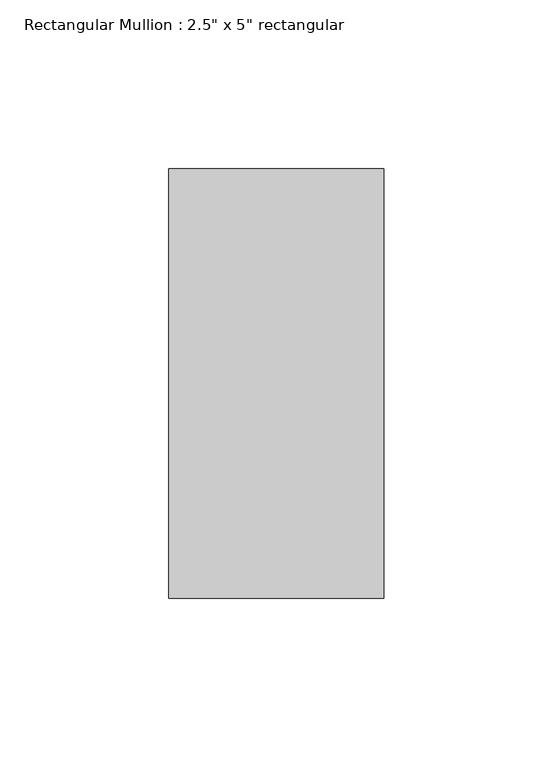
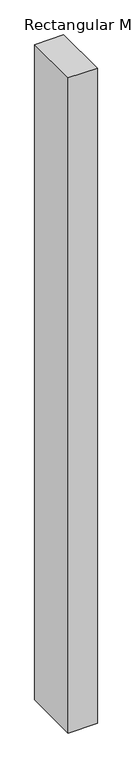
"""IFC4 building model written with IfcOpenShell, lengths in millimetres: member geometry."""

from ifc_helpers import new_model, si_unit, frame, origin, place, context, project, spatial, polyline, outline, extrude, source, transform, mapped, element, save


def member_7f309565(model_context):
    return source(origin(), model_context, "Body", "SweptSolid", [
        extrude(outline(polyline([(31.75, 63.5), (31.75, -63.5), (-31.75, -63.5), (-31.75, 63.5), (31.75, 63.5)])), frame((0.0, 0.0, -1513.5761917), z_axis=(0.0, 0.0, 1.0), x_axis=(1.0, 0.0, 0.0)), (0.0, 0.0, 1.0), 1513.5761917),
    ])


if __name__ == "__main__":
    model = new_model("IFC4")
    model_context = context("Model", 3, world=origin())
    ifc_project = project(units=[si_unit("LENGTHUNIT", "METRE", prefix="MILLI")], contexts=[model_context])
    site = spatial("IfcSite", under=ifc_project)
    building = spatial("IfcBuilding", under=site)
    placement = place(None, origin())
    member_shape = member_7f309565(model_context)
    element("IfcMember", 1, ObjectType="Rectangular Mullion : 2.5\" x 5\" rectangular", at=placement, inside=building, context=model_context, shape_type="MappedRepresentation", body=[
        mapped(member_shape, transform((0.0, 0.0, 0.0), x_axis=(1.0, 0.0, 0.0), y_axis=(0.0, 1.0, 0.0), z_axis=(0.0, 0.0, 1.0))),
    ])
    save(model, "model.ifc")

# Revit data of these elements
# Type "Rectangular Mullion : 2.5\" x 5\" rectangular"
#   built-in parameter 1007304 = 0.416667 (stored number, unit not read)
#   built-in parameter 1007301 = 0.104167 (stored number, unit not read)
#   built-in parameter 1007300 = 0.104167 (stored number, unit not read)
# Element 1 (IfcMember, "Rectangular Mullion : 2.5\" x 5\" rectangular")
#   Materials on its faces: "Aluminum"
# Materials
#   "Aluminum": class "Metal", colour RGB 247 247 247, transparency 0, Description = "Aluminum 6061", Cost = 0
